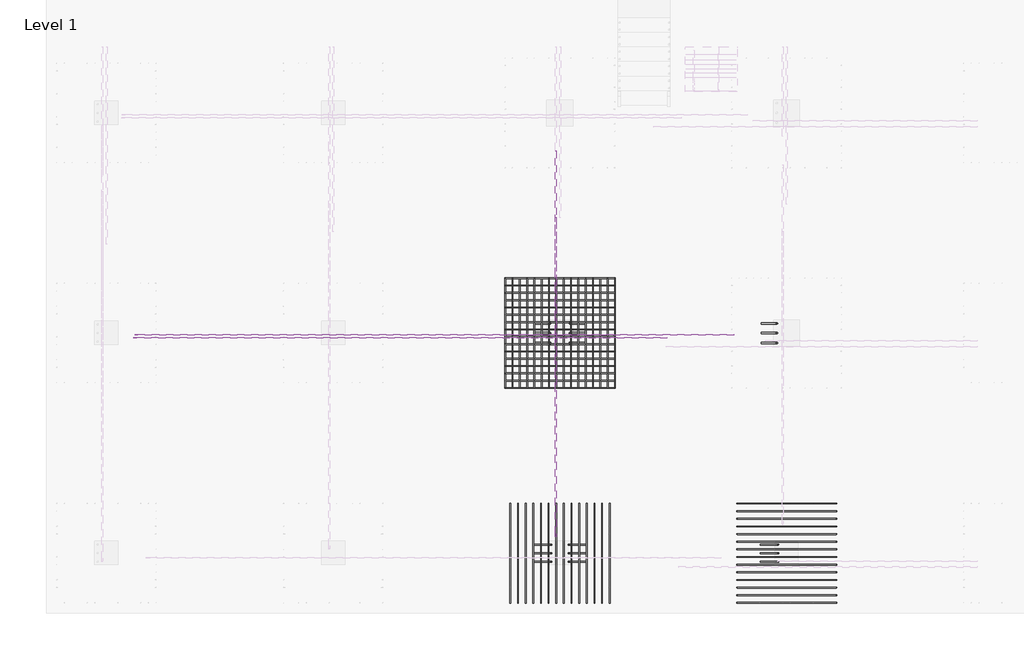
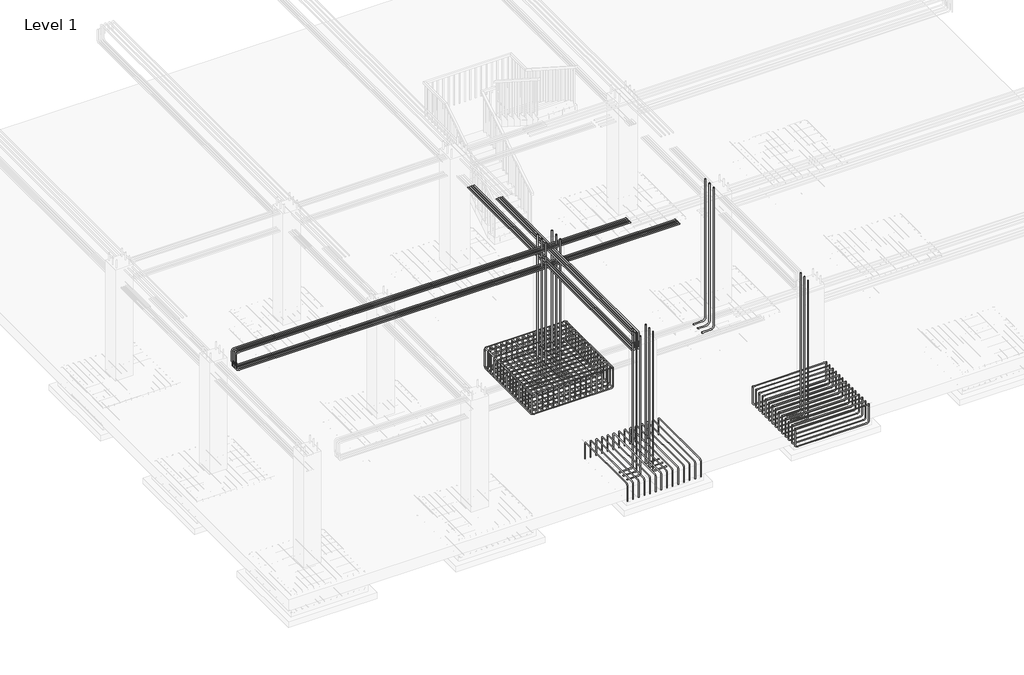
# One storey, part 5 of 17: 21 reinforcing bars.
"""IFC4 building model written with IfcOpenShell, lengths in millimetres."""

from ifc_helpers import new_model, si_unit, point, frame, origin, place, context, project, spatial, polyline, circle_curve, trimmed, segment, composite_curve, source, transform, mapped, element, save
from ifc_brep_helpers import swept_disk

model = new_model("IFC4")

# Units and contexts
model_context = context("Model", 3, world=origin())
ifc_project = project(units=[si_unit("LENGTHUNIT", "METRE", prefix="MILLI")], contexts=[model_context])

# Site, building, storey
site = spatial("IfcSite", under=ifc_project)
building = spatial("IfcBuilding", under=site)
storey = spatial("IfcBuildingStorey", under=building, Name="Level 1", Elevation=0.0)

# Reinforcing bars
placement = place(None, origin())
reinforcing_bar_shape = source(origin(), model_context, "Body", "SolidModel", [
    swept_disk(composite_curve([segment(polyline([(-4996.3632003, -3580.990543, -504.0), (-4996.3632003, -3580.990543, -96.0)]), True, "CONTINUOUS"), segment(trimmed(circle_curve(frame((-4996.3632003, -3628.990543, -96.0), z_axis=(1.0, 0.0, 0.0), x_axis=(0.0, 48.0, 0.0)), 48.0), [point((-4996.3632003, -3580.990543, -96.0))], [point((-4996.3632003, -3628.990543, -48.0))], True, "CARTESIAN"), True, "CONTINUOUS"), segment(polyline([(-4996.3632003, -3628.990543, -48.0), (-4996.3632003, -5436.990543, -48.0)]), True, "CONTINUOUS"), segment(trimmed(circle_curve(frame((-4996.3632003, -5436.990543, -96.0), z_axis=(1.0, 0.0, 0.0), x_axis=(0.0, 0.0, 48.0)), 48.0), [point((-4996.3632003, -5436.990543, -48.0))], [point((-4996.3632003, -5484.990543, -96.0))], True, "CARTESIAN"), True, "CONTINUOUS"), segment(polyline([(-4996.3632003, -5484.990543, -96.0), (-4996.3632003, -5484.990543, -504.0)]), True, "CONTINUOUS")], self_intersect=False), 8.0),
])
element("IfcReinforcingBar", 1, at=placement, inside=storey, context=model_context, shape_type="MappedRepresentation", body=[
    mapped(reinforcing_bar_shape, transform((0.0, 0.0, 0.0), x_axis=(1.0, 0.0, 0.0), y_axis=(0.0, 1.0, 0.0), z_axis=(0.0, 0.0, 1.0))),
    mapped(reinforcing_bar_shape, transform((146.4615385, 0.0, 0.0), x_axis=(1.0, 0.0, 0.0), y_axis=(0.0, 1.0, 0.0), z_axis=(0.0, 0.0, 1.0))),
    mapped(reinforcing_bar_shape, transform((292.9230769, 0.0, 0.0), x_axis=(1.0, 0.0, 0.0), y_axis=(0.0, 1.0, 0.0), z_axis=(0.0, 0.0, 1.0))),
    mapped(reinforcing_bar_shape, transform((439.3846154, 0.0, 0.0), x_axis=(1.0, 0.0, 0.0), y_axis=(0.0, 1.0, 0.0), z_axis=(0.0, 0.0, 1.0))),
    mapped(reinforcing_bar_shape, transform((585.8461538, 0.0, 0.0), x_axis=(1.0, 0.0, 0.0), y_axis=(0.0, 1.0, 0.0), z_axis=(0.0, 0.0, 1.0))),
    mapped(reinforcing_bar_shape, transform((732.3076923, 0.0, 0.0), x_axis=(1.0, 0.0, 0.0), y_axis=(0.0, 1.0, 0.0), z_axis=(0.0, 0.0, 1.0))),
    mapped(reinforcing_bar_shape, transform((878.7692308, 0.0, 0.0), x_axis=(1.0, 0.0, 0.0), y_axis=(0.0, 1.0, 0.0), z_axis=(0.0, 0.0, 1.0))),
    mapped(reinforcing_bar_shape, transform((1025.2307692, 0.0, 0.0), x_axis=(1.0, 0.0, 0.0), y_axis=(0.0, 1.0, 0.0), z_axis=(0.0, 0.0, 1.0))),
    mapped(reinforcing_bar_shape, transform((1171.6923077, 0.0, 0.0), x_axis=(1.0, 0.0, 0.0), y_axis=(0.0, 1.0, 0.0), z_axis=(0.0, 0.0, 1.0))),
    mapped(reinforcing_bar_shape, transform((1318.1538462, 0.0, 0.0), x_axis=(1.0, 0.0, 0.0), y_axis=(0.0, 1.0, 0.0), z_axis=(0.0, 0.0, 1.0))),
    mapped(reinforcing_bar_shape, transform((1464.6153846, 0.0, 0.0), x_axis=(1.0, 0.0, 0.0), y_axis=(0.0, 1.0, 0.0), z_axis=(0.0, 0.0, 1.0))),
    mapped(reinforcing_bar_shape, transform((1611.0769231, 0.0, 0.0), x_axis=(1.0, 0.0, 0.0), y_axis=(0.0, 1.0, 0.0), z_axis=(0.0, 0.0, 1.0))),
    mapped(reinforcing_bar_shape, transform((1757.5384615, 0.0, 0.0), x_axis=(1.0, 0.0, 0.0), y_axis=(0.0, 1.0, 0.0), z_axis=(0.0, 0.0, 1.0))),
    mapped(reinforcing_bar_shape, transform((1904.0, 0.0, 0.0), x_axis=(1.0, 0.0, 0.0), y_axis=(0.0, 1.0, 0.0), z_axis=(0.0, 0.0, 1.0))),
])
reinforcing_bar_2_shape = source(origin(), model_context, "Body", "SolidModel", [
    swept_disk(composite_curve([segment(polyline([(-4556.9785849, -4367.490543, -550.0), (-4259.8632003, -4367.490543, -550.0)]), True, "CONTINUOUS"), segment(trimmed(circle_curve(frame((-4259.8632003, -4367.490543, -500.0), z_axis=(0.0, -1.0, 0.0), x_axis=(0.0, 0.0, -50.0)), 50.0), [point((-4259.8632003, -4367.490543, -550.0))], [point((-4209.8632003, -4367.490543, -500.0))], True, "CARTESIAN"), True, "CONTINUOUS"), segment(polyline([(-4209.8632003, -4367.490543, -500.0), (-4209.8632003, -4367.490543, 3260.0)]), True, "CONTINUOUS")], self_intersect=False), 10.0),
])
element("IfcReinforcingBar", 2, at=placement, inside=storey, context=model_context, shape_type="MappedRepresentation", body=[
    mapped(reinforcing_bar_2_shape, transform((0.0, 0.0, 0.0), x_axis=(1.0, 0.0, 0.0), y_axis=(0.0, 1.0, 0.0), z_axis=(0.0, 0.0, 1.0))),
    mapped(reinforcing_bar_2_shape, transform((0.0, -165.5, 0.0), x_axis=(1.0, 0.0, 0.0), y_axis=(0.0, 1.0, 0.0), z_axis=(0.0, 0.0, 1.0))),
    mapped(reinforcing_bar_2_shape, transform((0.0, -331.0, 0.0), x_axis=(1.0, 0.0, 0.0), y_axis=(0.0, 1.0, 0.0), z_axis=(0.0, 0.0, 1.0))),
])
reinforcing_bar_3_shape = source(origin(), model_context, "Body", "SolidModel", [
    swept_disk(composite_curve([segment(polyline([(-3531.7478157, -4698.490543, -550.0), (-3828.8632003, -4698.490543, -550.0)]), True, "CONTINUOUS"), segment(trimmed(circle_curve(frame((-3828.8632003, -4698.490543, -500.0), z_axis=(0.0, 1.0, 0.0), x_axis=(0.0, 0.0, -50.0)), 50.0), [point((-3828.8632003, -4698.490543, -550.0))], [point((-3878.8632003, -4698.490543, -500.0))], True, "CARTESIAN"), True, "CONTINUOUS"), segment(polyline([(-3878.8632003, -4698.490543, -500.0), (-3878.8632003, -4698.490543, 3260.0)]), True, "CONTINUOUS")], self_intersect=False), 10.0),
])
element("IfcReinforcingBar", 3, at=placement, inside=storey, context=model_context, shape_type="MappedRepresentation", body=[
    mapped(reinforcing_bar_3_shape, transform((0.0, 0.0, 0.0), x_axis=(1.0, 0.0, 0.0), y_axis=(0.0, 1.0, 0.0), z_axis=(0.0, 0.0, 1.0))),
    mapped(reinforcing_bar_3_shape, transform((0.0, 165.5, 0.0), x_axis=(1.0, 0.0, 0.0), y_axis=(0.0, 1.0, 0.0), z_axis=(0.0, 0.0, 1.0))),
    mapped(reinforcing_bar_3_shape, transform((0.0, 331.0, 0.0), x_axis=(1.0, 0.0, 0.0), y_axis=(0.0, 1.0, 0.0), z_axis=(0.0, 0.0, 1.0))),
])
reinforcing_bar_4_shape = source(origin(), model_context, "Body", "SolidModel", [
    swept_disk(composite_curve([segment(polyline([(-651.3632003, -3580.990543, -40.0), (-651.3632003, -3580.990543, -504.0)]), True, "CONTINUOUS"), segment(trimmed(circle_curve(frame((-603.3632003, -3580.990543, -504.0), z_axis=(0.0, -1.0, 0.0), x_axis=(-48.0, 0.0, 0.0)), 48.0), [point((-651.3632003, -3580.990543, -504.0))], [point((-603.3632003, -3580.990543, -552.0))], True, "CARTESIAN"), True, "CONTINUOUS"), segment(polyline([(-603.3632003, -3580.990543, -552.0), (1204.6367997, -3580.990543, -552.0)]), True, "CONTINUOUS"), segment(trimmed(circle_curve(frame((1204.6367997, -3580.990543, -504.0), z_axis=(0.0, -1.0, 0.0), x_axis=(0.0, 0.0, -48.0)), 48.0), [point((1204.6367997, -3580.990543, -552.0))], [point((1252.6367997, -3580.990543, -504.0))], True, "CARTESIAN"), True, "CONTINUOUS"), segment(polyline([(1252.6367997, -3580.990543, -504.0), (1252.6367997, -3580.990543, -40.0)]), True, "CONTINUOUS")], self_intersect=False), 8.0),
])
element("IfcReinforcingBar", 4, at=placement, inside=storey, context=model_context, shape_type="MappedRepresentation", body=[
    mapped(reinforcing_bar_4_shape, transform((0.0, 0.0, 0.0), x_axis=(1.0, 0.0, 0.0), y_axis=(0.0, 1.0, 0.0), z_axis=(0.0, 0.0, 1.0))),
    mapped(reinforcing_bar_4_shape, transform((0.0, -146.4615385, 0.0), x_axis=(1.0, 0.0, 0.0), y_axis=(0.0, 1.0, 0.0), z_axis=(0.0, 0.0, 1.0))),
    mapped(reinforcing_bar_4_shape, transform((0.0, -292.9230769, 0.0), x_axis=(1.0, 0.0, 0.0), y_axis=(0.0, 1.0, 0.0), z_axis=(0.0, 0.0, 1.0))),
    mapped(reinforcing_bar_4_shape, transform((0.0, -439.3846154, 0.0), x_axis=(1.0, 0.0, 0.0), y_axis=(0.0, 1.0, 0.0), z_axis=(0.0, 0.0, 1.0))),
    mapped(reinforcing_bar_4_shape, transform((0.0, -585.8461538, 0.0), x_axis=(1.0, 0.0, 0.0), y_axis=(0.0, 1.0, 0.0), z_axis=(0.0, 0.0, 1.0))),
    mapped(reinforcing_bar_4_shape, transform((0.0, -732.3076923, 0.0), x_axis=(1.0, 0.0, 0.0), y_axis=(0.0, 1.0, 0.0), z_axis=(0.0, 0.0, 1.0))),
    mapped(reinforcing_bar_4_shape, transform((0.0, -878.7692308, 0.0), x_axis=(1.0, 0.0, 0.0), y_axis=(0.0, 1.0, 0.0), z_axis=(0.0, 0.0, 1.0))),
    mapped(reinforcing_bar_4_shape, transform((0.0, -1025.2307692, 0.0), x_axis=(1.0, 0.0, 0.0), y_axis=(0.0, 1.0, 0.0), z_axis=(0.0, 0.0, 1.0))),
    mapped(reinforcing_bar_4_shape, transform((0.0, -1171.6923077, 0.0), x_axis=(1.0, 0.0, 0.0), y_axis=(0.0, 1.0, 0.0), z_axis=(0.0, 0.0, 1.0))),
    mapped(reinforcing_bar_4_shape, transform((0.0, -1318.1538462, 0.0), x_axis=(1.0, 0.0, 0.0), y_axis=(0.0, 1.0, 0.0), z_axis=(0.0, 0.0, 1.0))),
    mapped(reinforcing_bar_4_shape, transform((0.0, -1464.6153846, 0.0), x_axis=(1.0, 0.0, 0.0), y_axis=(0.0, 1.0, 0.0), z_axis=(0.0, 0.0, 1.0))),
    mapped(reinforcing_bar_4_shape, transform((0.0, -1611.0769231, 0.0), x_axis=(1.0, 0.0, 0.0), y_axis=(0.0, 1.0, 0.0), z_axis=(0.0, 0.0, 1.0))),
    mapped(reinforcing_bar_4_shape, transform((0.0, -1757.5384615, 0.0), x_axis=(1.0, 0.0, 0.0), y_axis=(0.0, 1.0, 0.0), z_axis=(0.0, 0.0, 1.0))),
    mapped(reinforcing_bar_4_shape, transform((0.0, -1904.0, 0.0), x_axis=(1.0, 0.0, 0.0), y_axis=(0.0, 1.0, 0.0), z_axis=(0.0, 0.0, 1.0))),
])
reinforcing_bar_5_shape = source(origin(), model_context, "Body", "SolidModel", [
    swept_disk(composite_curve([segment(polyline([(-651.3632003, -5484.990543, -504.0), (-651.3632003, -5484.990543, -96.0)]), True, "CONTINUOUS"), segment(trimmed(circle_curve(frame((-603.3632003, -5484.990543, -96.0), z_axis=(0.0, 1.0, 0.0), x_axis=(-48.0, 0.0, 0.0)), 48.0), [point((-651.3632003, -5484.990543, -96.0))], [point((-603.3632003, -5484.990543, -48.0))], True, "CARTESIAN"), True, "CONTINUOUS"), segment(polyline([(-603.3632003, -5484.990543, -48.0), (1204.6367997, -5484.990543, -48.0)]), True, "CONTINUOUS"), segment(trimmed(circle_curve(frame((1204.6367997, -5484.990543, -96.0), z_axis=(0.0, 1.0, 0.0), x_axis=(0.0, 0.0, 48.0)), 48.0), [point((1204.6367997, -5484.990543, -48.0))], [point((1252.6367997, -5484.990543, -96.0))], True, "CARTESIAN"), True, "CONTINUOUS"), segment(polyline([(1252.6367997, -5484.990543, -96.0), (1252.6367997, -5484.990543, -504.0)]), True, "CONTINUOUS")], self_intersect=False), 8.0),
])
element("IfcReinforcingBar", 5, at=placement, inside=storey, context=model_context, shape_type="MappedRepresentation", body=[
    mapped(reinforcing_bar_5_shape, transform((0.0, 0.0, 0.0), x_axis=(1.0, 0.0, 0.0), y_axis=(0.0, 1.0, 0.0), z_axis=(0.0, 0.0, 1.0))),
    mapped(reinforcing_bar_5_shape, transform((0.0, 146.4615385, 0.0), x_axis=(1.0, 0.0, 0.0), y_axis=(0.0, 1.0, 0.0), z_axis=(0.0, 0.0, 1.0))),
    mapped(reinforcing_bar_5_shape, transform((0.0, 292.9230769, 0.0), x_axis=(1.0, 0.0, 0.0), y_axis=(0.0, 1.0, 0.0), z_axis=(0.0, 0.0, 1.0))),
    mapped(reinforcing_bar_5_shape, transform((0.0, 439.3846154, 0.0), x_axis=(1.0, 0.0, 0.0), y_axis=(0.0, 1.0, 0.0), z_axis=(0.0, 0.0, 1.0))),
    mapped(reinforcing_bar_5_shape, transform((0.0, 585.8461538, 0.0), x_axis=(1.0, 0.0, 0.0), y_axis=(0.0, 1.0, 0.0), z_axis=(0.0, 0.0, 1.0))),
    mapped(reinforcing_bar_5_shape, transform((0.0, 732.3076923, 0.0), x_axis=(1.0, 0.0, 0.0), y_axis=(0.0, 1.0, 0.0), z_axis=(0.0, 0.0, 1.0))),
    mapped(reinforcing_bar_5_shape, transform((0.0, 878.7692308, 0.0), x_axis=(1.0, 0.0, 0.0), y_axis=(0.0, 1.0, 0.0), z_axis=(0.0, 0.0, 1.0))),
    mapped(reinforcing_bar_5_shape, transform((0.0, 1025.2307692, 0.0), x_axis=(1.0, 0.0, 0.0), y_axis=(0.0, 1.0, 0.0), z_axis=(0.0, 0.0, 1.0))),
    mapped(reinforcing_bar_5_shape, transform((0.0, 1171.6923077, 0.0), x_axis=(1.0, 0.0, 0.0), y_axis=(0.0, 1.0, 0.0), z_axis=(0.0, 0.0, 1.0))),
    mapped(reinforcing_bar_5_shape, transform((0.0, 1318.1538462, 0.0), x_axis=(1.0, 0.0, 0.0), y_axis=(0.0, 1.0, 0.0), z_axis=(0.0, 0.0, 1.0))),
    mapped(reinforcing_bar_5_shape, transform((0.0, 1464.6153846, 0.0), x_axis=(1.0, 0.0, 0.0), y_axis=(0.0, 1.0, 0.0), z_axis=(0.0, 0.0, 1.0))),
    mapped(reinforcing_bar_5_shape, transform((0.0, 1611.0769231, 0.0), x_axis=(1.0, 0.0, 0.0), y_axis=(0.0, 1.0, 0.0), z_axis=(0.0, 0.0, 1.0))),
    mapped(reinforcing_bar_5_shape, transform((0.0, 1757.5384615, 0.0), x_axis=(1.0, 0.0, 0.0), y_axis=(0.0, 1.0, 0.0), z_axis=(0.0, 0.0, 1.0))),
    mapped(reinforcing_bar_5_shape, transform((0.0, 1904.0, 0.0), x_axis=(1.0, 0.0, 0.0), y_axis=(0.0, 1.0, 0.0), z_axis=(0.0, 0.0, 1.0))),
])
reinforcing_bar_6_shape = source(origin(), model_context, "Body", "SolidModel", [
    swept_disk(composite_curve([segment(polyline([(-211.9785849, -4367.490543, -550.0), (85.1367997, -4367.490543, -550.0)]), True, "CONTINUOUS"), segment(trimmed(circle_curve(frame((85.1367997, -4367.490543, -500.0), z_axis=(0.0, -1.0, 0.0), x_axis=(0.0, 0.0, -50.0)), 50.0), [point((85.1367997, -4367.490543, -550.0))], [point((135.1367997, -4367.490543, -500.0))], True, "CARTESIAN"), True, "CONTINUOUS"), segment(polyline([(135.1367997, -4367.490543, -500.0), (135.1367997, -4367.490543, 3260.0)]), True, "CONTINUOUS")], self_intersect=False), 10.0),
])
element("IfcReinforcingBar", 6, at=placement, inside=storey, context=model_context, shape_type="MappedRepresentation", body=[
    mapped(reinforcing_bar_6_shape, transform((0.0, 0.0, 0.0), x_axis=(1.0, 0.0, 0.0), y_axis=(0.0, 1.0, 0.0), z_axis=(0.0, 0.0, 1.0))),
    mapped(reinforcing_bar_6_shape, transform((0.0, -165.5, 0.0), x_axis=(1.0, 0.0, 0.0), y_axis=(0.0, 1.0, 0.0), z_axis=(0.0, 0.0, 1.0))),
    mapped(reinforcing_bar_6_shape, transform((0.0, -331.0, 0.0), x_axis=(1.0, 0.0, 0.0), y_axis=(0.0, 1.0, 0.0), z_axis=(0.0, 0.0, 1.0))),
])
reinforcing_bar_7_shape = source(origin(), model_context, "Body", "SolidModel", [
    swept_disk(composite_curve([segment(polyline([(-5096.3632003, 736.009457, -140.0), (-5096.3632003, 736.009457, -554.0)]), True, "CONTINUOUS"), segment(trimmed(circle_curve(frame((-5048.3632003, 736.009457, -554.0), z_axis=(0.0, -1.0, 0.0), x_axis=(-48.0, 0.0, 0.0)), 48.0), [point((-5096.3632003, 736.009457, -554.0))], [point((-5048.3632003, 736.009457, -602.0))], True, "CARTESIAN"), True, "CONTINUOUS"), segment(polyline([(-5048.3632003, 736.009457, -602.0), (-3040.3632003, 736.009457, -602.0)]), True, "CONTINUOUS"), segment(trimmed(circle_curve(frame((-3040.3632003, 736.009457, -554.0), z_axis=(0.0, -1.0, 0.0), x_axis=(0.0, 0.0, -48.0)), 48.0), [point((-3040.3632003, 736.009457, -602.0))], [point((-2992.3632003, 736.009457, -554.0))], True, "CARTESIAN"), True, "CONTINUOUS"), segment(polyline([(-2992.3632003, 736.009457, -554.0), (-2992.3632003, 736.009457, -140.0)]), True, "CONTINUOUS")], self_intersect=False), 8.0),
])
element("IfcReinforcingBar", 7, at=placement, inside=storey, context=model_context, shape_type="MappedRepresentation", body=[
    mapped(reinforcing_bar_7_shape, transform((0.0, 0.0, 0.0), x_axis=(1.0, 0.0, 0.0), y_axis=(0.0, 1.0, 0.0), z_axis=(0.0, 0.0, 1.0))),
    mapped(reinforcing_bar_7_shape, transform((0.0, -140.2666667, 0.0), x_axis=(1.0, 0.0, 0.0), y_axis=(0.0, 1.0, 0.0), z_axis=(0.0, 0.0, 1.0))),
    mapped(reinforcing_bar_7_shape, transform((0.0, -280.5333333, 0.0), x_axis=(1.0, 0.0, 0.0), y_axis=(0.0, 1.0, 0.0), z_axis=(0.0, 0.0, 1.0))),
    mapped(reinforcing_bar_7_shape, transform((0.0, -420.8, 0.0), x_axis=(1.0, 0.0, 0.0), y_axis=(0.0, 1.0, 0.0), z_axis=(0.0, 0.0, 1.0))),
    mapped(reinforcing_bar_7_shape, transform((0.0, -561.0666667, 0.0), x_axis=(1.0, 0.0, 0.0), y_axis=(0.0, 1.0, 0.0), z_axis=(0.0, 0.0, 1.0))),
    mapped(reinforcing_bar_7_shape, transform((0.0, -701.3333333, 0.0), x_axis=(1.0, 0.0, 0.0), y_axis=(0.0, 1.0, 0.0), z_axis=(0.0, 0.0, 1.0))),
    mapped(reinforcing_bar_7_shape, transform((0.0, -841.6, 0.0), x_axis=(1.0, 0.0, 0.0), y_axis=(0.0, 1.0, 0.0), z_axis=(0.0, 0.0, 1.0))),
    mapped(reinforcing_bar_7_shape, transform((0.0, -981.8666667, 0.0), x_axis=(1.0, 0.0, 0.0), y_axis=(0.0, 1.0, 0.0), z_axis=(0.0, 0.0, 1.0))),
    mapped(reinforcing_bar_7_shape, transform((0.0, -1122.1333333, 0.0), x_axis=(1.0, 0.0, 0.0), y_axis=(0.0, 1.0, 0.0), z_axis=(0.0, 0.0, 1.0))),
    mapped(reinforcing_bar_7_shape, transform((0.0, -1262.4, 0.0), x_axis=(1.0, 0.0, 0.0), y_axis=(0.0, 1.0, 0.0), z_axis=(0.0, 0.0, 1.0))),
    mapped(reinforcing_bar_7_shape, transform((0.0, -1402.6666667, 0.0), x_axis=(1.0, 0.0, 0.0), y_axis=(0.0, 1.0, 0.0), z_axis=(0.0, 0.0, 1.0))),
    mapped(reinforcing_bar_7_shape, transform((0.0, -1542.9333333, 0.0), x_axis=(1.0, 0.0, 0.0), y_axis=(0.0, 1.0, 0.0), z_axis=(0.0, 0.0, 1.0))),
    mapped(reinforcing_bar_7_shape, transform((0.0, -1683.2, 0.0), x_axis=(1.0, 0.0, 0.0), y_axis=(0.0, 1.0, 0.0), z_axis=(0.0, 0.0, 1.0))),
    mapped(reinforcing_bar_7_shape, transform((0.0, -1823.4666667, 0.0), x_axis=(1.0, 0.0, 0.0), y_axis=(0.0, 1.0, 0.0), z_axis=(0.0, 0.0, 1.0))),
    mapped(reinforcing_bar_7_shape, transform((0.0, -1963.7333333, 0.0), x_axis=(1.0, 0.0, 0.0), y_axis=(0.0, 1.0, 0.0), z_axis=(0.0, 0.0, 1.0))),
    mapped(reinforcing_bar_7_shape, transform((0.0, -2104.0, 0.0), x_axis=(1.0, 0.0, 0.0), y_axis=(0.0, 1.0, 0.0), z_axis=(0.0, 0.0, 1.0))),
])
reinforcing_bar_8_shape = source(origin(), model_context, "Body", "SolidModel", [
    swept_disk(composite_curve([segment(polyline([(-5096.3632003, -1367.990543, -554.0), (-5096.3632003, -1367.990543, -96.0)]), True, "CONTINUOUS"), segment(trimmed(circle_curve(frame((-5048.3632003, -1367.990543, -96.0), z_axis=(0.0, 1.0, 0.0), x_axis=(-48.0, 0.0, 0.0)), 48.0), [point((-5096.3632003, -1367.990543, -96.0))], [point((-5048.3632003, -1367.990543, -48.0))], True, "CARTESIAN"), True, "CONTINUOUS"), segment(polyline([(-5048.3632003, -1367.990543, -48.0), (-3040.3632003, -1367.990543, -48.0)]), True, "CONTINUOUS"), segment(trimmed(circle_curve(frame((-3040.3632003, -1367.990543, -96.0), z_axis=(0.0, 1.0, 0.0), x_axis=(0.0, 0.0, 48.0)), 48.0), [point((-3040.3632003, -1367.990543, -48.0))], [point((-2992.3632003, -1367.990543, -96.0))], True, "CARTESIAN"), True, "CONTINUOUS"), segment(polyline([(-2992.3632003, -1367.990543, -96.0), (-2992.3632003, -1367.990543, -554.0)]), True, "CONTINUOUS")], self_intersect=False), 8.0),
])
element("IfcReinforcingBar", 8, at=placement, inside=storey, context=model_context, shape_type="MappedRepresentation", body=[
    mapped(reinforcing_bar_8_shape, transform((0.0, 0.0, 0.0), x_axis=(1.0, 0.0, 0.0), y_axis=(0.0, 1.0, 0.0), z_axis=(0.0, 0.0, 1.0))),
    mapped(reinforcing_bar_8_shape, transform((0.0, 140.2666667, 0.0), x_axis=(1.0, 0.0, 0.0), y_axis=(0.0, 1.0, 0.0), z_axis=(0.0, 0.0, 1.0))),
    mapped(reinforcing_bar_8_shape, transform((0.0, 280.5333333, 0.0), x_axis=(1.0, 0.0, 0.0), y_axis=(0.0, 1.0, 0.0), z_axis=(0.0, 0.0, 1.0))),
    mapped(reinforcing_bar_8_shape, transform((0.0, 420.8, 0.0), x_axis=(1.0, 0.0, 0.0), y_axis=(0.0, 1.0, 0.0), z_axis=(0.0, 0.0, 1.0))),
    mapped(reinforcing_bar_8_shape, transform((0.0, 561.0666667, 0.0), x_axis=(1.0, 0.0, 0.0), y_axis=(0.0, 1.0, 0.0), z_axis=(0.0, 0.0, 1.0))),
    mapped(reinforcing_bar_8_shape, transform((0.0, 701.3333333, 0.0), x_axis=(1.0, 0.0, 0.0), y_axis=(0.0, 1.0, 0.0), z_axis=(0.0, 0.0, 1.0))),
    mapped(reinforcing_bar_8_shape, transform((0.0, 841.6, 0.0), x_axis=(1.0, 0.0, 0.0), y_axis=(0.0, 1.0, 0.0), z_axis=(0.0, 0.0, 1.0))),
    mapped(reinforcing_bar_8_shape, transform((0.0, 981.8666667, 0.0), x_axis=(1.0, 0.0, 0.0), y_axis=(0.0, 1.0, 0.0), z_axis=(0.0, 0.0, 1.0))),
    mapped(reinforcing_bar_8_shape, transform((0.0, 1122.1333333, 0.0), x_axis=(1.0, 0.0, 0.0), y_axis=(0.0, 1.0, 0.0), z_axis=(0.0, 0.0, 1.0))),
    mapped(reinforcing_bar_8_shape, transform((0.0, 1262.4, 0.0), x_axis=(1.0, 0.0, 0.0), y_axis=(0.0, 1.0, 0.0), z_axis=(0.0, 0.0, 1.0))),
    mapped(reinforcing_bar_8_shape, transform((0.0, 1402.6666667, 0.0), x_axis=(1.0, 0.0, 0.0), y_axis=(0.0, 1.0, 0.0), z_axis=(0.0, 0.0, 1.0))),
    mapped(reinforcing_bar_8_shape, transform((0.0, 1542.9333333, 0.0), x_axis=(1.0, 0.0, 0.0), y_axis=(0.0, 1.0, 0.0), z_axis=(0.0, 0.0, 1.0))),
    mapped(reinforcing_bar_8_shape, transform((0.0, 1683.2, 0.0), x_axis=(1.0, 0.0, 0.0), y_axis=(0.0, 1.0, 0.0), z_axis=(0.0, 0.0, 1.0))),
    mapped(reinforcing_bar_8_shape, transform((0.0, 1823.4666667, 0.0), x_axis=(1.0, 0.0, 0.0), y_axis=(0.0, 1.0, 0.0), z_axis=(0.0, 0.0, 1.0))),
    mapped(reinforcing_bar_8_shape, transform((0.0, 1963.7333333, 0.0), x_axis=(1.0, 0.0, 0.0), y_axis=(0.0, 1.0, 0.0), z_axis=(0.0, 0.0, 1.0))),
    mapped(reinforcing_bar_8_shape, transform((0.0, 2104.0, 0.0), x_axis=(1.0, 0.0, 0.0), y_axis=(0.0, 1.0, 0.0), z_axis=(0.0, 0.0, 1.0))),
])
reinforcing_bar_9_shape = source(origin(), model_context, "Body", "SolidModel", [
    swept_disk(composite_curve([segment(polyline([(-2992.3632003, 736.009457, -100.0), (-2992.3632003, 736.009457, -554.0)]), True, "CONTINUOUS"), segment(trimmed(circle_curve(frame((-2992.3632003, 688.009457, -554.0), z_axis=(-1.0, 0.0, 0.0), x_axis=(0.0, 48.0, 0.0)), 48.0), [point((-2992.3632003, 736.009457, -554.0))], [point((-2992.3632003, 688.009457, -602.0))], True, "CARTESIAN"), True, "CONTINUOUS"), segment(polyline([(-2992.3632003, 688.009457, -602.0), (-2992.3632003, -1319.990543, -602.0)]), True, "CONTINUOUS"), segment(trimmed(circle_curve(frame((-2992.3632003, -1319.990543, -554.0), z_axis=(-1.0, 0.0, 0.0), x_axis=(0.0, 0.0, -48.0)), 48.0), [point((-2992.3632003, -1319.990543, -602.0))], [point((-2992.3632003, -1367.990543, -554.0))], True, "CARTESIAN"), True, "CONTINUOUS"), segment(polyline([(-2992.3632003, -1367.990543, -554.0), (-2992.3632003, -1367.990543, -100.0)]), True, "CONTINUOUS")], self_intersect=False), 8.0),
])
element("IfcReinforcingBar", 9, at=placement, inside=storey, context=model_context, shape_type="MappedRepresentation", body=[
    mapped(reinforcing_bar_9_shape, transform((0.0, 0.0, 0.0), x_axis=(1.0, 0.0, 0.0), y_axis=(0.0, 1.0, 0.0), z_axis=(0.0, 0.0, 1.0))),
    mapped(reinforcing_bar_9_shape, transform((-140.2666667, 0.0, 0.0), x_axis=(1.0, 0.0, 0.0), y_axis=(0.0, 1.0, 0.0), z_axis=(0.0, 0.0, 1.0))),
    mapped(reinforcing_bar_9_shape, transform((-280.5333333, 0.0, 0.0), x_axis=(1.0, 0.0, 0.0), y_axis=(0.0, 1.0, 0.0), z_axis=(0.0, 0.0, 1.0))),
    mapped(reinforcing_bar_9_shape, transform((-420.8, 0.0, 0.0), x_axis=(1.0, 0.0, 0.0), y_axis=(0.0, 1.0, 0.0), z_axis=(0.0, 0.0, 1.0))),
    mapped(reinforcing_bar_9_shape, transform((-561.0666667, 0.0, 0.0), x_axis=(1.0, 0.0, 0.0), y_axis=(0.0, 1.0, 0.0), z_axis=(0.0, 0.0, 1.0))),
    mapped(reinforcing_bar_9_shape, transform((-701.3333333, 0.0, 0.0), x_axis=(1.0, 0.0, 0.0), y_axis=(0.0, 1.0, 0.0), z_axis=(0.0, 0.0, 1.0))),
    mapped(reinforcing_bar_9_shape, transform((-841.6, 0.0, 0.0), x_axis=(1.0, 0.0, 0.0), y_axis=(0.0, 1.0, 0.0), z_axis=(0.0, 0.0, 1.0))),
    mapped(reinforcing_bar_9_shape, transform((-981.8666667, 0.0, 0.0), x_axis=(1.0, 0.0, 0.0), y_axis=(0.0, 1.0, 0.0), z_axis=(0.0, 0.0, 1.0))),
    mapped(reinforcing_bar_9_shape, transform((-1122.1333333, 0.0, 0.0), x_axis=(1.0, 0.0, 0.0), y_axis=(0.0, 1.0, 0.0), z_axis=(0.0, 0.0, 1.0))),
    mapped(reinforcing_bar_9_shape, transform((-1262.4, 0.0, 0.0), x_axis=(1.0, 0.0, 0.0), y_axis=(0.0, 1.0, 0.0), z_axis=(0.0, 0.0, 1.0))),
    mapped(reinforcing_bar_9_shape, transform((-1402.6666667, 0.0, 0.0), x_axis=(1.0, 0.0, 0.0), y_axis=(0.0, 1.0, 0.0), z_axis=(0.0, 0.0, 1.0))),
    mapped(reinforcing_bar_9_shape, transform((-1542.9333333, 0.0, 0.0), x_axis=(1.0, 0.0, 0.0), y_axis=(0.0, 1.0, 0.0), z_axis=(0.0, 0.0, 1.0))),
    mapped(reinforcing_bar_9_shape, transform((-1683.2, 0.0, 0.0), x_axis=(1.0, 0.0, 0.0), y_axis=(0.0, 1.0, 0.0), z_axis=(0.0, 0.0, 1.0))),
    mapped(reinforcing_bar_9_shape, transform((-1823.4666667, 0.0, 0.0), x_axis=(1.0, 0.0, 0.0), y_axis=(0.0, 1.0, 0.0), z_axis=(0.0, 0.0, 1.0))),
    mapped(reinforcing_bar_9_shape, transform((-1963.7333333, 0.0, 0.0), x_axis=(1.0, 0.0, 0.0), y_axis=(0.0, 1.0, 0.0), z_axis=(0.0, 0.0, 1.0))),
    mapped(reinforcing_bar_9_shape, transform((-2104.0, 0.0, 0.0), x_axis=(1.0, 0.0, 0.0), y_axis=(0.0, 1.0, 0.0), z_axis=(0.0, 0.0, 1.0))),
])
reinforcing_bar_10_shape = source(origin(), model_context, "Body", "SolidModel", [
    swept_disk(composite_curve([segment(polyline([(-5096.3632003, 736.009457, -560.0), (-5096.3632003, 736.009457, -96.0)]), True, "CONTINUOUS"), segment(trimmed(circle_curve(frame((-5096.3632003, 688.009457, -96.0), z_axis=(1.0, 0.0, 0.0), x_axis=(0.0, 48.0, 0.0)), 48.0), [point((-5096.3632003, 736.009457, -96.0))], [point((-5096.3632003, 688.009457, -48.0))], True, "CARTESIAN"), True, "CONTINUOUS"), segment(polyline([(-5096.3632003, 688.009457, -48.0), (-5096.3632003, -1319.990543, -48.0)]), True, "CONTINUOUS"), segment(trimmed(circle_curve(frame((-5096.3632003, -1319.990543, -96.0), z_axis=(1.0, 0.0, 0.0), x_axis=(0.0, 0.0, 48.0)), 48.0), [point((-5096.3632003, -1319.990543, -48.0))], [point((-5096.3632003, -1367.990543, -96.0))], True, "CARTESIAN"), True, "CONTINUOUS"), segment(polyline([(-5096.3632003, -1367.990543, -96.0), (-5096.3632003, -1367.990543, -560.0)]), True, "CONTINUOUS")], self_intersect=False), 8.0),
])
element("IfcReinforcingBar", 10, at=placement, inside=storey, context=model_context, shape_type="MappedRepresentation", body=[
    mapped(reinforcing_bar_10_shape, transform((0.0, 0.0, 0.0), x_axis=(1.0, 0.0, 0.0), y_axis=(0.0, 1.0, 0.0), z_axis=(0.0, 0.0, 1.0))),
    mapped(reinforcing_bar_10_shape, transform((140.2666667, 0.0, 0.0), x_axis=(1.0, 0.0, 0.0), y_axis=(0.0, 1.0, 0.0), z_axis=(0.0, 0.0, 1.0))),
    mapped(reinforcing_bar_10_shape, transform((280.5333333, 0.0, 0.0), x_axis=(1.0, 0.0, 0.0), y_axis=(0.0, 1.0, 0.0), z_axis=(0.0, 0.0, 1.0))),
    mapped(reinforcing_bar_10_shape, transform((420.8, 0.0, 0.0), x_axis=(1.0, 0.0, 0.0), y_axis=(0.0, 1.0, 0.0), z_axis=(0.0, 0.0, 1.0))),
    mapped(reinforcing_bar_10_shape, transform((561.0666667, 0.0, 0.0), x_axis=(1.0, 0.0, 0.0), y_axis=(0.0, 1.0, 0.0), z_axis=(0.0, 0.0, 1.0))),
    mapped(reinforcing_bar_10_shape, transform((701.3333333, 0.0, 0.0), x_axis=(1.0, 0.0, 0.0), y_axis=(0.0, 1.0, 0.0), z_axis=(0.0, 0.0, 1.0))),
    mapped(reinforcing_bar_10_shape, transform((841.6, 0.0, 0.0), x_axis=(1.0, 0.0, 0.0), y_axis=(0.0, 1.0, 0.0), z_axis=(0.0, 0.0, 1.0))),
    mapped(reinforcing_bar_10_shape, transform((981.8666667, 0.0, 0.0), x_axis=(1.0, 0.0, 0.0), y_axis=(0.0, 1.0, 0.0), z_axis=(0.0, 0.0, 1.0))),
    mapped(reinforcing_bar_10_shape, transform((1122.1333333, 0.0, 0.0), x_axis=(1.0, 0.0, 0.0), y_axis=(0.0, 1.0, 0.0), z_axis=(0.0, 0.0, 1.0))),
    mapped(reinforcing_bar_10_shape, transform((1262.4, 0.0, 0.0), x_axis=(1.0, 0.0, 0.0), y_axis=(0.0, 1.0, 0.0), z_axis=(0.0, 0.0, 1.0))),
    mapped(reinforcing_bar_10_shape, transform((1402.6666667, 0.0, 0.0), x_axis=(1.0, 0.0, 0.0), y_axis=(0.0, 1.0, 0.0), z_axis=(0.0, 0.0, 1.0))),
    mapped(reinforcing_bar_10_shape, transform((1542.9333333, 0.0, 0.0), x_axis=(1.0, 0.0, 0.0), y_axis=(0.0, 1.0, 0.0), z_axis=(0.0, 0.0, 1.0))),
    mapped(reinforcing_bar_10_shape, transform((1683.2, 0.0, 0.0), x_axis=(1.0, 0.0, 0.0), y_axis=(0.0, 1.0, 0.0), z_axis=(0.0, 0.0, 1.0))),
    mapped(reinforcing_bar_10_shape, transform((1823.4666667, 0.0, 0.0), x_axis=(1.0, 0.0, 0.0), y_axis=(0.0, 1.0, 0.0), z_axis=(0.0, 0.0, 1.0))),
    mapped(reinforcing_bar_10_shape, transform((1963.7333333, 0.0, 0.0), x_axis=(1.0, 0.0, 0.0), y_axis=(0.0, 1.0, 0.0), z_axis=(0.0, 0.0, 1.0))),
    mapped(reinforcing_bar_10_shape, transform((2104.0, 0.0, 0.0), x_axis=(1.0, 0.0, 0.0), y_axis=(0.0, 1.0, 0.0), z_axis=(0.0, 0.0, 1.0))),
])
reinforcing_bar_11_shape = source(origin(), model_context, "Body", "SolidModel", [
    swept_disk(composite_curve([segment(polyline([(-4535.2965336, -128.190543, -597.3), (-4322.3632003, -128.190543, -597.3)]), True, "CONTINUOUS"), segment(trimmed(circle_curve(frame((-4322.3632003, -128.190543, -507.1), z_axis=(0.0, -1.0, 0.0), x_axis=(0.0, 0.0, -90.19999999999993)), 90.2), [point((-4322.3632003, -128.190543, -597.3))], [point((-4232.1632003, -128.190543, -507.1))], True, "CARTESIAN"), True, "CONTINUOUS"), segment(polyline([(-4232.1632003, -128.190543, -507.1), (-4232.1632003, -128.190543, 3270.0)]), True, "CONTINUOUS")], self_intersect=False), 12.7),
])
element("IfcReinforcingBar", 11, at=placement, inside=storey, context=model_context, shape_type="MappedRepresentation", body=[
    mapped(reinforcing_bar_11_shape, transform((0.0, 0.0, 0.0), x_axis=(1.0, 0.0, 0.0), y_axis=(0.0, 1.0, 0.0), z_axis=(0.0, 0.0, 1.0))),
    mapped(reinforcing_bar_11_shape, transform((0.0, -187.8, 0.0), x_axis=(1.0, 0.0, 0.0), y_axis=(0.0, 1.0, 0.0), z_axis=(0.0, 0.0, 1.0))),
    mapped(reinforcing_bar_11_shape, transform((0.0, -375.6, 0.0), x_axis=(1.0, 0.0, 0.0), y_axis=(0.0, 1.0, 0.0), z_axis=(0.0, 0.0, 1.0))),
])
reinforcing_bar_12_shape = source(origin(), model_context, "Body", "SolidModel", [
    swept_disk(composite_curve([segment(polyline([(-3553.429867, -503.790543, -597.3), (-3766.3632003, -503.790543, -597.3)]), True, "CONTINUOUS"), segment(trimmed(circle_curve(frame((-3766.3632003, -503.790543, -507.1), z_axis=(0.0, 1.0, 0.0), x_axis=(0.0, 0.0, -90.19999999999993)), 90.2), [point((-3766.3632003, -503.790543, -597.3))], [point((-3856.5632003, -503.790543, -507.1))], True, "CARTESIAN"), True, "CONTINUOUS"), segment(polyline([(-3856.5632003, -503.790543, -507.1), (-3856.5632003, -503.790543, 3250.0)]), True, "CONTINUOUS")], self_intersect=False), 12.7),
])
element("IfcReinforcingBar", 12, at=placement, inside=storey, context=model_context, shape_type="MappedRepresentation", body=[
    mapped(reinforcing_bar_12_shape, transform((0.0, 0.0, 0.0), x_axis=(1.0, 0.0, 0.0), y_axis=(0.0, 1.0, 0.0), z_axis=(0.0, 0.0, 1.0))),
    mapped(reinforcing_bar_12_shape, transform((0.0, 187.8, 0.0), x_axis=(1.0, 0.0, 0.0), y_axis=(0.0, 1.0, 0.0), z_axis=(0.0, 0.0, 1.0))),
    mapped(reinforcing_bar_12_shape, transform((0.0, 375.6, 0.0), x_axis=(1.0, 0.0, 0.0), y_axis=(0.0, 1.0, 0.0), z_axis=(0.0, 0.0, 1.0))),
])
reinforcing_bar_13_shape = source(origin(), model_context, "Body", "SolidModel", [
    swept_disk(composite_curve([segment(polyline([(-190.2965336, -128.190543, -597.3), (22.6367997, -128.190543, -597.3)]), True, "CONTINUOUS"), segment(trimmed(circle_curve(frame((22.6367997, -128.190543, -507.1), z_axis=(0.0, -1.0, 0.0), x_axis=(0.0, 0.0, -90.19999999999993)), 90.2), [point((22.6367997, -128.190543, -597.3))], [point((112.8367997, -128.190543, -507.1))], True, "CARTESIAN"), True, "CONTINUOUS"), segment(polyline([(112.8367997, -128.190543, -507.1), (112.8367997, -128.190543, 3270.0)]), True, "CONTINUOUS")], self_intersect=False), 12.7),
])
element("IfcReinforcingBar", 13, at=placement, inside=storey, context=model_context, shape_type="MappedRepresentation", body=[
    mapped(reinforcing_bar_13_shape, transform((0.0, 0.0, 0.0), x_axis=(1.0, 0.0, 0.0), y_axis=(0.0, 1.0, 0.0), z_axis=(0.0, 0.0, 1.0))),
    mapped(reinforcing_bar_13_shape, transform((0.0, -187.8, 0.0), x_axis=(1.0, 0.0, 0.0), y_axis=(0.0, 1.0, 0.0), z_axis=(0.0, 0.0, 1.0))),
    mapped(reinforcing_bar_13_shape, transform((0.0, -375.6, 0.0), x_axis=(1.0, 0.0, 0.0), y_axis=(0.0, 1.0, 0.0), z_axis=(0.0, 0.0, 1.0))),
])
reinforcing_bar_14_shape = source(origin(), model_context, "Body", "SolidModel", [
    swept_disk(composite_curve([segment(polyline([(-712.4632003, -406.490543, 2507.5), (-12136.7632003, -406.490543, 2507.5)]), True, "CONTINUOUS"), segment(trimmed(circle_curve(frame((-12136.7632003, -406.490543, 2557.5), z_axis=(0.0, 1.0, 0.0), x_axis=(0.0, 0.0, -50.0)), 50.0), [point((-12136.7632003, -406.490543, 2507.5))], [point((-12186.7632003, -406.490543, 2557.5))], True, "CARTESIAN"), True, "CONTINUOUS"), segment(polyline([(-12186.7632003, -406.490543, 2557.5), (-12186.7632003, -406.490543, 2707.4)]), True, "CONTINUOUS")], self_intersect=False), 10.0),
])
element("IfcReinforcingBar", 14, at=placement, inside=storey, context=model_context, shape_type="MappedRepresentation", body=[
    mapped(reinforcing_bar_14_shape, transform((0.0, 0.0, 0.0), x_axis=(1.0, 0.0, 0.0), y_axis=(0.0, 1.0, 0.0), z_axis=(0.0, 0.0, 1.0))),
    mapped(reinforcing_bar_14_shape, transform((0.0, 60.3333333, 0.0), x_axis=(1.0, 0.0, 0.0), y_axis=(0.0, 1.0, 0.0), z_axis=(0.0, 0.0, 1.0))),
    mapped(reinforcing_bar_14_shape, transform((0.0, 120.6666667, 0.0), x_axis=(1.0, 0.0, 0.0), y_axis=(0.0, 1.0, 0.0), z_axis=(0.0, 0.0, 1.0))),
    mapped(reinforcing_bar_14_shape, transform((0.0, 181.0, 0.0), x_axis=(1.0, 0.0, 0.0), y_axis=(0.0, 1.0, 0.0), z_axis=(0.0, 0.0, 1.0))),
])
reinforcing_bar_15_shape = source(origin(), model_context, "Body", "SolidModel", [
    swept_disk(composite_curve([segment(polyline([(-1987.4632003, -225.490543, 2988.5), (-12151.5132003, -225.490543, 2988.5)]), True, "CONTINUOUS"), segment(trimmed(circle_curve(frame((-12151.5132003, -225.490543, 2938.5), z_axis=(0.0, -1.0, 0.0), x_axis=(0.0, 0.0, 50.0)), 50.0), [point((-12151.5132003, -225.490543, 2988.5))], [point((-12201.5132003, -225.490543, 2938.5))], True, "CARTESIAN"), True, "CONTINUOUS"), segment(polyline([(-12201.5132003, -225.490543, 2938.5), (-12201.5132003, -225.490543, 2648.0)]), True, "CONTINUOUS")], self_intersect=False), 10.0),
])
element("IfcReinforcingBar", 15, at=placement, inside=storey, context=model_context, shape_type="MappedRepresentation", body=[
    mapped(reinforcing_bar_15_shape, transform((0.0, 0.0, 0.0), x_axis=(1.0, 0.0, 0.0), y_axis=(0.0, 1.0, 0.0), z_axis=(0.0, 0.0, 1.0))),
    mapped(reinforcing_bar_15_shape, transform((0.0, -60.3333333, 0.0), x_axis=(1.0, 0.0, 0.0), y_axis=(0.0, 1.0, 0.0), z_axis=(0.0, 0.0, 1.0))),
    mapped(reinforcing_bar_15_shape, transform((0.0, -120.6666667, 0.0), x_axis=(1.0, 0.0, 0.0), y_axis=(0.0, 1.0, 0.0), z_axis=(0.0, 0.0, 1.0))),
    mapped(reinforcing_bar_15_shape, transform((0.0, -181.0, 0.0), x_axis=(1.0, 0.0, 0.0), y_axis=(0.0, 1.0, 0.0), z_axis=(0.0, 0.0, 1.0))),
])
reinforcing_bar_16_shape = source(origin(), model_context, "Body", "SolidModel", [
    swept_disk(composite_curve([segment(polyline([(-3964.3632003, 3175.609457, 2518.0), (-3964.3632003, -4157.590543, 2518.0)]), True, "CONTINUOUS"), segment(trimmed(circle_curve(frame((-3964.3632003, -4157.590543, 2568.0), z_axis=(-1.0, 0.0, 0.0), x_axis=(0.0, 0.0, -50.0)), 50.0), [point((-3964.3632003, -4157.590543, 2518.0))], [point((-3964.3632003, -4207.590543, 2568.0))], True, "CARTESIAN"), True, "CONTINUOUS"), segment(polyline([(-3964.3632003, -4207.590543, 2568.0), (-3964.3632003, -4207.590543, 2748.0)]), True, "CONTINUOUS")], self_intersect=False), 10.0),
])
element("IfcReinforcingBar", 16, at=placement, inside=storey, context=model_context, shape_type="MappedRepresentation", body=[
    mapped(reinforcing_bar_16_shape, transform((0.0, 0.0, 0.0), x_axis=(1.0, 0.0, 0.0), y_axis=(0.0, 1.0, 0.0), z_axis=(0.0, 0.0, 1.0))),
    mapped(reinforcing_bar_16_shape, transform((-53.3333333, 0.0, 0.0), x_axis=(1.0, 0.0, 0.0), y_axis=(0.0, 1.0, 0.0), z_axis=(0.0, 0.0, 1.0))),
    mapped(reinforcing_bar_16_shape, transform((-106.6666667, 0.0, 0.0), x_axis=(1.0, 0.0, 0.0), y_axis=(0.0, 1.0, 0.0), z_axis=(0.0, 0.0, 1.0))),
    mapped(reinforcing_bar_16_shape, transform((-160.0, 0.0, 0.0), x_axis=(1.0, 0.0, 0.0), y_axis=(0.0, 1.0, 0.0), z_axis=(0.0, 0.0, 1.0))),
])
reinforcing_bar_17_shape = source(origin(), model_context, "Body", "SolidModel", [
    swept_disk(composite_curve([segment(polyline([(-4124.3632003, 1900.609457, 2978.0), (-4124.3632003, -4163.090543, 2978.0)]), True, "CONTINUOUS"), segment(trimmed(circle_curve(frame((-4124.3632003, -4163.090543, 2928.0), z_axis=(1.0, 0.0, 0.0), x_axis=(0.0, 0.0, 50.0)), 50.0), [point((-4124.3632003, -4163.090543, 2978.0))], [point((-4124.3632003, -4213.090543, 2928.0))], True, "CARTESIAN"), True, "CONTINUOUS"), segment(polyline([(-4124.3632003, -4213.090543, 2928.0), (-4124.3632003, -4213.090543, 2608.0)]), True, "CONTINUOUS")], self_intersect=False), 10.0),
])
element("IfcReinforcingBar", 17, at=placement, inside=storey, context=model_context, shape_type="MappedRepresentation", body=[
    mapped(reinforcing_bar_17_shape, transform((0.0, 0.0, 0.0), x_axis=(1.0, 0.0, 0.0), y_axis=(0.0, 1.0, 0.0), z_axis=(0.0, 0.0, 1.0))),
    mapped(reinforcing_bar_17_shape, transform((53.3333333, 0.0, 0.0), x_axis=(1.0, 0.0, 0.0), y_axis=(0.0, 1.0, 0.0), z_axis=(0.0, 0.0, 1.0))),
    mapped(reinforcing_bar_17_shape, transform((106.6666667, 0.0, 0.0), x_axis=(1.0, 0.0, 0.0), y_axis=(0.0, 1.0, 0.0), z_axis=(0.0, 0.0, 1.0))),
    mapped(reinforcing_bar_17_shape, transform((160.0, 0.0, 0.0), x_axis=(1.0, 0.0, 0.0), y_axis=(0.0, 1.0, 0.0), z_axis=(0.0, 0.0, 1.0))),
])
reinforcing_bar_18_shape = source(origin(), model_context, "Body", "SolidModel", [
    swept_disk(composite_curve([segment(polyline([(-712.4632003, -406.490543, 2507.5), (-12136.7632003, -406.490543, 2507.5)]), True, "CONTINUOUS"), segment(trimmed(circle_curve(frame((-12136.7632003, -406.490543, 2557.5), z_axis=(0.0, 1.0, 0.0), x_axis=(0.0, 0.0, -50.0)), 50.0), [point((-12136.7632003, -406.490543, 2507.5))], [point((-12186.7632003, -406.490543, 2557.5))], True, "CARTESIAN"), True, "CONTINUOUS"), segment(polyline([(-12186.7632003, -406.490543, 2557.5), (-12186.7632003, -406.490543, 2707.4)]), True, "CONTINUOUS")], self_intersect=False), 10.0),
])
element("IfcReinforcingBar", 18, at=placement, inside=storey, context=model_context, shape_type="MappedRepresentation", body=[
    mapped(reinforcing_bar_18_shape, transform((0.0, 0.0, 0.0), x_axis=(1.0, 0.0, 0.0), y_axis=(0.0, 1.0, 0.0), z_axis=(0.0, 0.0, 1.0))),
    mapped(reinforcing_bar_18_shape, transform((0.0, 60.3333333, 0.0), x_axis=(1.0, 0.0, 0.0), y_axis=(0.0, 1.0, 0.0), z_axis=(0.0, 0.0, 1.0))),
    mapped(reinforcing_bar_18_shape, transform((0.0, 120.6666667, 0.0), x_axis=(1.0, 0.0, 0.0), y_axis=(0.0, 1.0, 0.0), z_axis=(0.0, 0.0, 1.0))),
    mapped(reinforcing_bar_18_shape, transform((0.0, 181.0, 0.0), x_axis=(1.0, 0.0, 0.0), y_axis=(0.0, 1.0, 0.0), z_axis=(0.0, 0.0, 1.0))),
])
reinforcing_bar_19_shape = source(origin(), model_context, "Body", "SolidModel", [
    swept_disk(composite_curve([segment(polyline([(-1987.4632003, -225.490543, 2988.5), (-12151.5132003, -225.490543, 2988.5)]), True, "CONTINUOUS"), segment(trimmed(circle_curve(frame((-12151.5132003, -225.490543, 2938.5), z_axis=(0.0, -1.0, 0.0), x_axis=(0.0, 0.0, 50.0)), 50.0), [point((-12151.5132003, -225.490543, 2988.5))], [point((-12201.5132003, -225.490543, 2938.5))], True, "CARTESIAN"), True, "CONTINUOUS"), segment(polyline([(-12201.5132003, -225.490543, 2938.5), (-12201.5132003, -225.490543, 2648.0)]), True, "CONTINUOUS")], self_intersect=False), 10.0),
])
element("IfcReinforcingBar", 19, at=placement, inside=storey, context=model_context, shape_type="MappedRepresentation", body=[
    mapped(reinforcing_bar_19_shape, transform((0.0, 0.0, 0.0), x_axis=(1.0, 0.0, 0.0), y_axis=(0.0, 1.0, 0.0), z_axis=(0.0, 0.0, 1.0))),
    mapped(reinforcing_bar_19_shape, transform((0.0, -60.3333333, 0.0), x_axis=(1.0, 0.0, 0.0), y_axis=(0.0, 1.0, 0.0), z_axis=(0.0, 0.0, 1.0))),
    mapped(reinforcing_bar_19_shape, transform((0.0, -120.6666667, 0.0), x_axis=(1.0, 0.0, 0.0), y_axis=(0.0, 1.0, 0.0), z_axis=(0.0, 0.0, 1.0))),
    mapped(reinforcing_bar_19_shape, transform((0.0, -181.0, 0.0), x_axis=(1.0, 0.0, 0.0), y_axis=(0.0, 1.0, 0.0), z_axis=(0.0, 0.0, 1.0))),
])
reinforcing_bar_20_shape = source(origin(), model_context, "Body", "SolidModel", [
    swept_disk(composite_curve([segment(polyline([(-3964.3632003, 3175.609457, 2518.0), (-3964.3632003, -4157.590543, 2518.0)]), True, "CONTINUOUS"), segment(trimmed(circle_curve(frame((-3964.3632003, -4157.590543, 2568.0), z_axis=(-1.0, 0.0, 0.0), x_axis=(0.0, 0.0, -50.0)), 50.0), [point((-3964.3632003, -4157.590543, 2518.0))], [point((-3964.3632003, -4207.590543, 2568.0))], True, "CARTESIAN"), True, "CONTINUOUS"), segment(polyline([(-3964.3632003, -4207.590543, 2568.0), (-3964.3632003, -4207.590543, 2748.0)]), True, "CONTINUOUS")], self_intersect=False), 10.0),
])
element("IfcReinforcingBar", 20, at=placement, inside=storey, context=model_context, shape_type="MappedRepresentation", body=[
    mapped(reinforcing_bar_20_shape, transform((0.0, 0.0, 0.0), x_axis=(1.0, 0.0, 0.0), y_axis=(0.0, 1.0, 0.0), z_axis=(0.0, 0.0, 1.0))),
    mapped(reinforcing_bar_20_shape, transform((-53.3333333, 0.0, 0.0), x_axis=(1.0, 0.0, 0.0), y_axis=(0.0, 1.0, 0.0), z_axis=(0.0, 0.0, 1.0))),
    mapped(reinforcing_bar_20_shape, transform((-106.6666667, 0.0, 0.0), x_axis=(1.0, 0.0, 0.0), y_axis=(0.0, 1.0, 0.0), z_axis=(0.0, 0.0, 1.0))),
    mapped(reinforcing_bar_20_shape, transform((-160.0, 0.0, 0.0), x_axis=(1.0, 0.0, 0.0), y_axis=(0.0, 1.0, 0.0), z_axis=(0.0, 0.0, 1.0))),
])
reinforcing_bar_21_shape = source(origin(), model_context, "Body", "SolidModel", [
    swept_disk(composite_curve([segment(polyline([(-4124.3632003, 1900.609457, 2978.0), (-4124.3632003, -4163.090543, 2978.0)]), True, "CONTINUOUS"), segment(trimmed(circle_curve(frame((-4124.3632003, -4163.090543, 2928.0), z_axis=(1.0, 0.0, 0.0), x_axis=(0.0, 0.0, 50.0)), 50.0), [point((-4124.3632003, -4163.090543, 2978.0))], [point((-4124.3632003, -4213.090543, 2928.0))], True, "CARTESIAN"), True, "CONTINUOUS"), segment(polyline([(-4124.3632003, -4213.090543, 2928.0), (-4124.3632003, -4213.090543, 2608.0)]), True, "CONTINUOUS")], self_intersect=False), 10.0),
])
element("IfcReinforcingBar", 21, at=placement, inside=storey, context=model_context, shape_type="MappedRepresentation", body=[
    mapped(reinforcing_bar_21_shape, transform((0.0, 0.0, 0.0), x_axis=(1.0, 0.0, 0.0), y_axis=(0.0, 1.0, 0.0), z_axis=(0.0, 0.0, 1.0))),
    mapped(reinforcing_bar_21_shape, transform((53.3333333, 0.0, 0.0), x_axis=(1.0, 0.0, 0.0), y_axis=(0.0, 1.0, 0.0), z_axis=(0.0, 0.0, 1.0))),
    mapped(reinforcing_bar_21_shape, transform((106.6666667, 0.0, 0.0), x_axis=(1.0, 0.0, 0.0), y_axis=(0.0, 1.0, 0.0), z_axis=(0.0, 0.0, 1.0))),
    mapped(reinforcing_bar_21_shape, transform((160.0, 0.0, 0.0), x_axis=(1.0, 0.0, 0.0), y_axis=(0.0, 1.0, 0.0), z_axis=(0.0, 0.0, 1.0))),
])

save(model, "model.ifc")

# Revit data of these elements
# Elements 1, 2, 3, 4, 5, 6, 7, 8, 9, 10, 11, 12, 13, 14, 15, 16, 17, 18, 19, 20, 21 (IfcReinforcingBar)
#   Phase Created = New Construction
